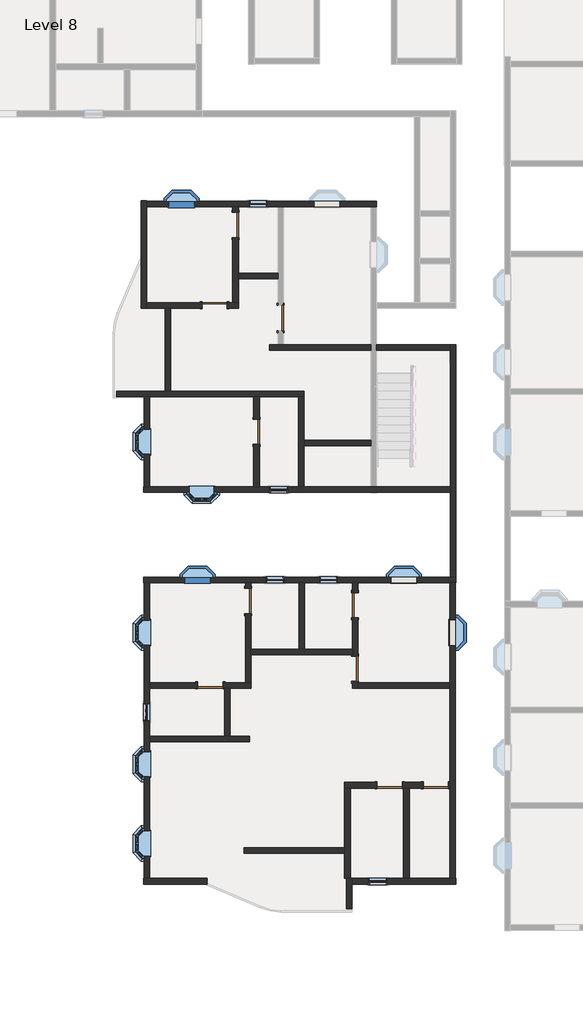
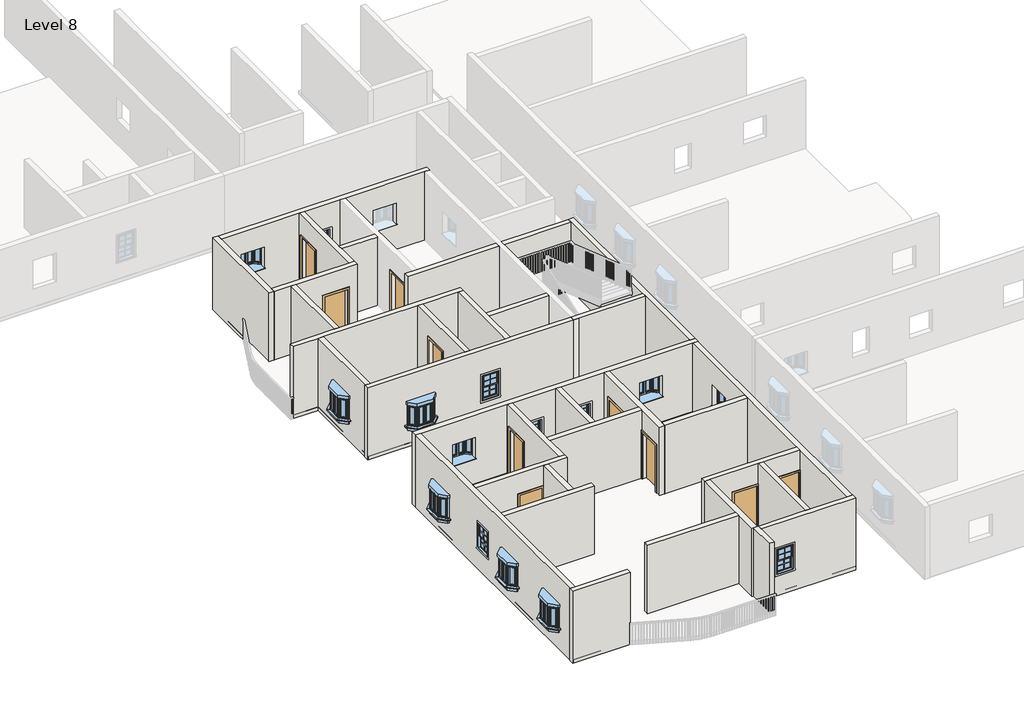
# One storey, part 1 of 14: 33 walls, 15 windows, 10 doors.
"""IFC4 building model written with IfcOpenShell, lengths in millimetres."""

from ifc_helpers import new_model, si_unit, frame, origin, place, context, project, spatial, polyline, outline, extrude, faceted_brep, transform, mapped, element, save
from components import door_54dd4da4, door_719f80de, window_910x910mm_67ef725a, window_8debb0fa

model = new_model("IFC4")

# Units and contexts
model_context = context("Model", 3, world=origin())
ifc_project = project(units=[si_unit("LENGTHUNIT", "METRE", prefix="MILLI")], contexts=[model_context])

# Site, building, storey
site = spatial("IfcSite", under=ifc_project)
building = spatial("IfcBuilding", under=site)
storey = spatial("IfcBuildingStorey", under=building, Name="Level 8", Elevation=21336.0)

# Doors
placement = place(None, origin())
door_shape = door_54dd4da4(model_context)
element("IfcDoor", 1, ObjectType="Single-Flush : 36\" x 84\"", at=placement, inside=storey, context=model_context, shape_type="MappedRepresentation", body=[
    mapped(door_shape, transform((-4626.037215, -17283.4916506, 21336.0), x_axis=(0.0, -1.0, 0.0), y_axis=(1.0, 0.0, 0.0), z_axis=(0.0, 0.0, 1.0))),
])
element("IfcDoor", 2, ObjectType="Single-Flush : 36\" x 84\"", at=placement, inside=storey, context=model_context, shape_type="MappedRepresentation", body=[
    mapped(door_shape, transform((-4626.037215, -14978.4416506, 21336.0), x_axis=(0.0, 1.0, 0.0), y_axis=(-1.0, 0.0, 0.0), z_axis=(0.0, 0.0, 1.0))),
])
element("IfcDoor", 3, ObjectType="Single-Flush : 36\" x 84\"", at=placement, inside=storey, context=model_context, shape_type="MappedRepresentation", body=[
    mapped(door_shape, transform((-9731.437215, -4100.8916506, 21336.0), x_axis=(1.0, 0.0, 0.0), y_axis=(0.0, 1.0, 0.0), z_axis=(0.0, 0.0, 1.0))),
])
element("IfcDoor", 4, ObjectType="Single-Flush : 36\" x 84\"", at=placement, inside=storey, context=model_context, shape_type="MappedRepresentation", body=[
    mapped(door_shape, transform((-7331.137215, -4558.0916506, 21336.0), x_axis=(0.0, -1.0, 0.0), y_axis=(1.0, 0.0, 0.0), z_axis=(0.0, 0.0, 1.0))),
])
door_2_shape = door_719f80de(model_context)
element("IfcDoor", 5, ObjectType="Single-Flush : 36\" x 84\"", at=placement, inside=storey, context=model_context, shape_type="MappedRepresentation", body=[
    mapped(door_2_shape, transform((-9883.837215, -17891.2072331, 21336.0), x_axis=(1.0, 0.0, 0.0), y_axis=(0.0, 1.0, 0.0), z_axis=(0.0, 0.0, 1.0))),
])
element("IfcDoor", 6, ObjectType="Single-Flush : 36\" x 84\"", at=placement, inside=storey, context=model_context, shape_type="MappedRepresentation", body=[
    mapped(door_2_shape, transform((-8512.237215, -14826.0416506, 21336.0), x_axis=(0.0, 1.0, 0.0), y_axis=(-1.0, 0.0, 0.0), z_axis=(0.0, 0.0, 1.0))),
])
element("IfcDoor", 7, ObjectType="Single-Flush : 36\" x 84\"", at=placement, inside=storey, context=model_context, shape_type="MappedRepresentation", body=[
    mapped(door_2_shape, transform((-8207.437215, -8691.9416506, 21336.0), x_axis=(0.0, 1.0, 0.0), y_axis=(-1.0, 0.0, 0.0), z_axis=(0.0, 0.0, 1.0))),
])
element("IfcDoor", 8, ObjectType="Single-Flush : 36\" x 84\"", at=placement, inside=storey, context=model_context, shape_type="MappedRepresentation", body=[
    mapped(door_2_shape, transform((-8969.437215, -1186.2416506, 21336.0), x_axis=(0.0, 1.0, 0.0), y_axis=(-1.0, 0.0, 0.0), z_axis=(0.0, 0.0, 1.0))),
])
element("IfcDoor", 9, ObjectType="Single-Flush : 36\" x 84\"", at=placement, inside=storey, context=model_context, shape_type="MappedRepresentation", body=[
    mapped(door_2_shape, transform((-3374.4891351, -21512.5916506, 21336.0), x_axis=(1.0, 0.0, 0.0), y_axis=(0.0, 1.0, 0.0), z_axis=(0.0, 0.0, 1.0))),
])
element("IfcDoor", 10, ObjectType="Single-Flush : 36\" x 84\"", at=placement, inside=storey, context=model_context, shape_type="MappedRepresentation", body=[
    mapped(door_2_shape, transform((-1698.0891351, -21512.5916506, 21336.0), x_axis=(1.0, 0.0, 0.0), y_axis=(0.0, 1.0, 0.0), z_axis=(0.0, 0.0, 1.0))),
])

# Walls
element("IfcWall", 11, ObjectType="4.5\" p", at=placement, inside=storey, context=model_context, shape_type="Brep", body=[
    faceted_brep([(-9426.637215, -17992.8072331, 23469.6), (-9426.637215, -17992.8072331, 21336.0), (-9375.837215, -17992.8072331, 21336.0), (-9172.637215, -17992.8072331, 21336.0), (-8410.637215, -17992.8072331, 21336.0), (-8410.637215, -17992.8072331, 24384.0), (-9172.637215, -17992.8072331, 24384.0), (-9375.837215, -17992.8072331, 24384.0), (-12087.287215, -17992.8072331, 24384.0), (-12087.287215, -17992.8072331, 21336.0), (-10341.037215, -17992.8072331, 21336.0), (-10341.037215, -17992.8072331, 23469.6), (-8410.637215, -17789.6072331, 21336.0), (-8613.837215, -17789.6072331, 21336.0), (-9426.637215, -17789.6072331, 21336.0), (-9426.637215, -17789.6072331, 23469.6), (-10341.037215, -17789.6072331, 23469.6), (-10341.037215, -17789.6072331, 21336.0), (-12087.287215, -17789.6072331, 21336.0), (-12087.287215, -17789.6072331, 24384.0), (-8613.837215, -17789.6072331, 24384.0), (-8410.637215, -17789.6072331, 24384.0)], [[[0, 1, 2, 3, 4, 5, 6, 7, 8, 9, 10, 11]], [[12, 13, 14, 15, 16, 17, 18, 19, 20, 21]], [[10, 9, 18, 17]], [[4, 3, 2, 1, 14, 13, 12]], [[8, 7, 6, 5, 21, 20, 19]], [[9, 8, 19, 18]], [[5, 4, 12, 21]], [[15, 14, 1, 0]], [[16, 15, 0, 11]], [[17, 16, 11, 10]]]),
])
element("IfcWall", 12, ObjectType="4.5\" p", at=placement, inside=storey, context=model_context, shape_type="Brep", body=[
    faceted_brep([(-8410.637215, -14368.8416506, 23469.6), (-8410.637215, -14368.8416506, 21336.0), (-8410.637215, -14165.6416506, 21336.0), (-8410.637215, -14165.6416506, 24384.0), (-8410.637215, -16572.2916506, 24384.0), (-8410.637215, -16775.4916506, 24384.0), (-8410.637215, -17789.6072331, 24384.0), (-8410.637215, -17789.6072331, 21336.0), (-8410.637215, -16775.4916506, 21336.0), (-8410.637215, -16572.2916506, 21336.0), (-8410.637215, -15283.2416506, 21336.0), (-8410.637215, -15283.2416506, 23469.6), (-8613.837215, -14165.6416506, 21336.0), (-8613.837215, -14368.8416506, 21336.0), (-8613.837215, -14368.8416506, 23469.6), (-8613.837215, -15283.2416506, 23469.6), (-8613.837215, -15283.2416506, 21336.0), (-8613.837215, -17789.6072331, 21336.0), (-8613.837215, -17789.6072331, 24384.0), (-8613.837215, -14165.6416506, 24384.0)], [[[0, 1, 2, 3, 4, 5, 6, 7, 8, 9, 10, 11]], [[12, 13, 14, 15, 16, 17, 18, 19]], [[2, 1, 13, 12]], [[10, 9, 8, 7, 17, 16]], [[6, 5, 4, 3, 19, 18]], [[7, 6, 18, 17]], [[3, 2, 12, 19]], [[14, 13, 1, 0]], [[15, 14, 0, 11]], [[16, 15, 11, 10]]]),
])
element("IfcWall", 13, ObjectType="4.5\" p", at=placement, inside=storey, context=model_context, shape_type="Brep", body=[
    faceted_brep([(-8410.637215, -16775.4916506, 21336.0), (-4727.637215, -16775.4916506, 21336.0), (-4727.637215, -16775.4916506, 24384.0), (-8410.637215, -16775.4916506, 24384.0), (-8410.637215, -16572.2916506, 21336.0), (-8410.637215, -16572.2916506, 24384.0), (-6670.737215, -16572.2916506, 24384.0), (-6467.537215, -16572.2916506, 24384.0), (-4727.637215, -16572.2916506, 24384.0), (-4727.637215, -16572.2916506, 21336.0), (-6467.537215, -16572.2916506, 21336.0), (-6670.737215, -16572.2916506, 21336.0)], [[[0, 1, 2, 3]], [[4, 5, 6, 7, 8, 9, 10, 11]], [[1, 0, 4, 11, 10, 9]], [[3, 2, 8, 7, 6, 5]], [[0, 3, 5, 4]], [[2, 1, 9, 8]]]),
])
element("IfcWall", 14, ObjectType="4.5\" p", at=placement, inside=storey, context=model_context, shape_type="SweptSolid", body=[
    extrude(outline(polyline([(-6670.737215, -16572.2916506), (-6670.737215, -14165.6416506), (-6467.537215, -14165.6416506), (-6467.537215, -16572.2916506), (-6670.737215, -16572.2916506)])), frame((0.0, 0.0, 21336.0), z_axis=(0.0, 0.0, 1.0), x_axis=(1.0, 0.0, 0.0)), (0.0, 0.0, 1.0), 3048.0),
])
element("IfcWall", 15, ObjectType="4.5\" p", at=placement, inside=storey, context=model_context, shape_type="Brep", body=[
    faceted_brep([(-4727.637215, -14165.6416506, 21336.0), (-4727.637215, -14521.2416506, 21336.0), (-4727.637215, -14521.2416506, 23469.6), (-4727.637215, -15435.6416506, 23469.6), (-4727.637215, -15435.6416506, 21336.0), (-4727.637215, -16572.2916506, 21336.0), (-4727.637215, -16775.4916506, 21336.0), (-4727.637215, -16826.2916506, 21336.0), (-4727.637215, -16826.2916506, 23469.6), (-4727.637215, -17740.6916506, 23469.6), (-4727.637215, -17740.6916506, 21336.0), (-4727.637215, -17994.6916506, 21336.0), (-4727.637215, -17994.6916506, 24384.0), (-4727.637215, -16775.4916506, 24384.0), (-4727.637215, -16572.2916506, 24384.0), (-4727.637215, -14165.6416506, 24384.0), (-4524.437215, -14521.2416506, 23469.6), (-4524.437215, -14521.2416506, 21336.0), (-4524.437215, -14165.6416506, 21336.0), (-4524.437215, -14165.6416506, 24384.0), (-4524.437215, -17791.4916506, 24384.0), (-4524.437215, -17994.6916506, 24384.0), (-4524.437215, -17994.6916506, 21336.0), (-4524.437215, -17791.4916506, 21336.0), (-4524.437215, -17740.6916506, 21336.0), (-4524.437215, -17740.6916506, 23469.6), (-4524.437215, -16826.2916506, 23469.6), (-4524.437215, -16826.2916506, 21336.0), (-4524.437215, -15435.6416506, 21336.0), (-4524.437215, -15435.6416506, 23469.6)], [[[0, 1, 2, 3, 4, 5, 6, 7, 8, 9, 10, 11, 12, 13, 14, 15]], [[16, 17, 18, 19, 20, 21, 22, 23, 24, 25, 26, 27, 28, 29]], [[11, 10, 24, 23, 22]], [[28, 27, 7, 6, 5, 4]], [[18, 17, 1, 0]], [[15, 14, 13, 12, 21, 20, 19]], [[0, 15, 19, 18]], [[12, 11, 22, 21]], [[25, 24, 10, 9]], [[26, 25, 9, 8]], [[27, 26, 8, 7]], [[2, 1, 17, 16]], [[3, 2, 16, 29]], [[4, 3, 29, 28]]]),
])
element("IfcWall", 16, ObjectType="4.5\" p", at=placement, inside=storey, context=model_context, shape_type="SweptSolid", body=[
    extrude(outline(polyline([(-4524.437215, -17791.4916506), (-1190.0891351, -17791.4916506), (-1190.0891351, -17994.6916506), (-4524.437215, -17994.6916506), (-4524.437215, -17791.4916506)])), frame((0.0, 0.0, 21336.0), z_axis=(0.0, 0.0, 1.0), x_axis=(1.0, 0.0, 0.0)), (0.0, 0.0, 1.0), 3048.0),
])
element("IfcWall", 17, ObjectType="4.5\" p", at=placement, inside=storey, context=model_context, shape_type="SweptSolid", body=[
    extrude(outline(polyline([(-9375.837215, -19734.5916506), (-9375.837215, -17992.8072331), (-9172.637215, -17992.8072331), (-9172.637215, -19734.5916506), (-9375.837215, -19734.5916506)])), frame((0.0, 0.0, 21336.0), z_axis=(0.0, 0.0, 1.0), x_axis=(1.0, 0.0, 0.0)), (0.0, 0.0, 1.0), 3048.0),
])
element("IfcWall", 18, ObjectType="4.5\" p", at=placement, inside=storey, context=model_context, shape_type="Brep", body=[
    faceted_brep([(-12087.287215, -19937.7916506, 21336.0), (-8455.087215, -19937.7916506, 21336.0), (-8455.087215, -19937.7916506, 24384.0), (-12087.287215, -19937.7916506, 24384.0), (-12087.287215, -19734.5916506, 21336.0), (-12087.287215, -19734.5916506, 24384.0), (-9375.837215, -19734.5916506, 24384.0), (-9172.637215, -19734.5916506, 24384.0), (-8455.087215, -19734.5916506, 24384.0), (-8455.087215, -19734.5916506, 21336.0), (-9172.637215, -19734.5916506, 21336.0), (-9375.837215, -19734.5916506, 21336.0)], [[[0, 1, 2, 3]], [[4, 5, 6, 7, 8, 9, 10, 11]], [[1, 0, 4, 11, 10, 9]], [[2, 1, 9, 8]], [[3, 2, 8, 7, 6, 5]], [[0, 3, 5, 4]]]),
])
element("IfcWall", 19, ObjectType="4.5\" p", at=placement, inside=storey, context=model_context, shape_type="Brep", body=[
    faceted_brep([(-13293.787215, -7421.9416506, 21336.0), (-12290.487215, -7421.9416506, 21336.0), (-12087.287215, -7421.9416506, 21336.0), (-8309.037215, -7421.9416506, 21336.0), (-8105.837215, -7421.9416506, 21336.0), (-6689.787215, -7421.9416506, 21336.0), (-6486.587215, -7421.9416506, 21336.0), (-6486.587215, -7421.9416506, 24384.0), (-6689.787215, -7421.9416506, 24384.0), (-8105.837215, -7421.9416506, 24384.0), (-8309.037215, -7421.9416506, 24384.0), (-12087.287215, -7421.9416506, 24384.0), (-12290.487215, -7421.9416506, 24384.0), (-13293.787215, -7421.9416506, 24384.0), (-13293.787215, -7218.7416506, 21336.0), (-13293.787215, -7218.7416506, 24384.0), (-11528.487215, -7218.7416506, 24384.0), (-11325.287215, -7218.7416506, 24384.0), (-6486.587215, -7218.7416506, 24384.0), (-6486.587215, -7218.7416506, 21336.0), (-11325.287215, -7218.7416506, 21336.0), (-11528.487215, -7218.7416506, 21336.0)], [[[0, 1, 2, 3, 4, 5, 6, 7, 8, 9, 10, 11, 12, 13]], [[14, 15, 16, 17, 18, 19, 20, 21]], [[6, 5, 4, 3, 2, 1, 0, 14, 21, 20, 19]], [[13, 12, 11, 10, 9, 8, 7, 18, 17, 16, 15]], [[0, 13, 15, 14]], [[7, 6, 19, 18]]]),
])
element("IfcWall", 20, ObjectType="4.5\" p", at=placement, inside=storey, context=model_context, shape_type="Brep", body=[
    faceted_brep([(-12201.587215, -4202.4916506, 21336.0), (-12201.587215, -3999.2916506, 21336.0), (-12201.587215, -525.8416506, 21336.0), (-12201.587215, -322.6416506, 21336.0), (-12201.587215, -309.9416506, 21336.0), (-12201.587215, -309.9416506, 24384.0), (-12201.587215, -322.6416506, 24384.0), (-12201.587215, -525.8416506, 24384.0), (-12201.587215, -3999.2916506, 24384.0), (-12201.587215, -4202.4916506, 24384.0), (-12404.787215, -4202.4916506, 21336.0), (-12404.787215, -4202.4916506, 24384.0), (-12404.787215, -309.9416506, 24384.0), (-12404.787215, -309.9416506, 21336.0)], [[[0, 1, 2, 3, 4, 5, 6, 7, 8, 9]], [[10, 11, 12, 13]], [[4, 3, 2, 1, 0, 10, 13]], [[5, 4, 13, 12]], [[9, 8, 7, 6, 5, 12, 11]], [[0, 9, 11, 10]]]),
])
element("IfcWall", 21, ObjectType="4.5\" p", at=placement, inside=storey, context=model_context, shape_type="Brep", body=[
    faceted_brep([(-9274.237215, -4202.4916506, 23469.6), (-9274.237215, -4202.4916506, 21336.0), (-8867.837215, -4202.4916506, 21336.0), (-8867.837215, -4202.4916506, 24384.0), (-11325.287215, -4202.4916506, 24384.0), (-11528.487215, -4202.4916506, 24384.0), (-12201.587215, -4202.4916506, 24384.0), (-12201.587215, -4202.4916506, 21336.0), (-11528.487215, -4202.4916506, 21336.0), (-11325.287215, -4202.4916506, 21336.0), (-10188.637215, -4202.4916506, 21336.0), (-10188.637215, -4202.4916506, 23469.6), (-8867.837215, -3999.2916506, 21336.0), (-9071.037215, -3999.2916506, 21336.0), (-9274.237215, -3999.2916506, 21336.0), (-9274.237215, -3999.2916506, 23469.6), (-10188.637215, -3999.2916506, 23469.6), (-10188.637215, -3999.2916506, 21336.0), (-12201.587215, -3999.2916506, 21336.0), (-12201.587215, -3999.2916506, 24384.0), (-9071.037215, -3999.2916506, 24384.0), (-8867.837215, -3999.2916506, 24384.0)], [[[0, 1, 2, 3, 4, 5, 6, 7, 8, 9, 10, 11]], [[12, 13, 14, 15, 16, 17, 18, 19, 20, 21]], [[2, 1, 14, 13, 12]], [[10, 9, 8, 7, 18, 17]], [[6, 5, 4, 3, 21, 20, 19]], [[7, 6, 19, 18]], [[3, 2, 12, 21]], [[15, 14, 1, 0]], [[16, 15, 0, 11]], [[17, 16, 11, 10]]]),
])
element("IfcWall", 22, ObjectType="4.5\" p", at=placement, inside=storey, context=model_context, shape_type="Brep", body=[
    faceted_brep([(-8867.837215, -729.0416506, 23469.6), (-8867.837215, -729.0416506, 21336.0), (-8867.837215, -525.8416506, 21336.0), (-8867.837215, -525.8416506, 24384.0), (-8867.837215, -2932.4916506, 24384.0), (-8867.837215, -3135.6916506, 24384.0), (-8867.837215, -3999.2916506, 24384.0), (-8867.837215, -3999.2916506, 21336.0), (-8867.837215, -3135.6916506, 21336.0), (-8867.837215, -2932.4916506, 21336.0), (-8867.837215, -1643.4416506, 21336.0), (-8867.837215, -1643.4416506, 23469.6), (-9071.037215, -525.8416506, 21336.0), (-9071.037215, -729.0416506, 21336.0), (-9071.037215, -729.0416506, 23469.6), (-9071.037215, -1643.4416506, 23469.6), (-9071.037215, -1643.4416506, 21336.0), (-9071.037215, -3999.2916506, 21336.0), (-9071.037215, -3999.2916506, 24384.0), (-9071.037215, -525.8416506, 24384.0)], [[[0, 1, 2, 3, 4, 5, 6, 7, 8, 9, 10, 11]], [[12, 13, 14, 15, 16, 17, 18, 19]], [[2, 1, 13, 12]], [[10, 9, 8, 7, 17, 16]], [[6, 5, 4, 3, 19, 18]], [[7, 6, 18, 17]], [[3, 2, 12, 19]], [[14, 13, 1, 0]], [[15, 14, 0, 11]], [[16, 15, 11, 10]]]),
])
element("IfcWall", 23, ObjectType="4.5\" p", at=placement, inside=storey, context=model_context, shape_type="SweptSolid", body=[
    extrude(outline(polyline([(-7432.737215, -3135.6916506), (-8867.837215, -3135.6916506), (-8867.837215, -2932.4916506), (-7432.737215, -2932.4916506), (-7432.737215, -3135.6916506)])), frame((0.0, 0.0, 21336.0), z_axis=(0.0, 0.0, 1.0), x_axis=(1.0, 0.0, 0.0)), (0.0, 0.0, 1.0), 3048.0),
])
element("IfcWall", 24, ObjectType="4.5\" p", at=placement, inside=storey, context=model_context, shape_type="Brep", body=[
    faceted_brep([(-7731.187215, -5726.4916506, 24384.0), (-7731.187215, -5726.4916506, 21336.0), (-4060.887215, -5726.4916506, 21336.0), (-4060.887215, -5726.4916506, 24384.0), (-7731.187215, -5523.2916506, 21336.0), (-7731.187215, -5523.2916506, 24384.0), (-7432.737215, -5523.2916506, 24384.0), (-7229.537215, -5523.2916506, 24384.0), (-4060.887215, -5523.2916506, 24384.0), (-4060.887215, -5523.2916506, 21336.0), (-7229.537215, -5523.2916506, 21336.0), (-7432.737215, -5523.2916506, 21336.0)], [[[0, 1, 2, 3]], [[4, 5, 6, 7, 8, 9, 10, 11]], [[1, 4, 11, 10, 9, 2]], [[5, 0, 3, 8, 7, 6]], [[1, 0, 5, 4]], [[3, 2, 9, 8]]]),
    faceted_brep([(-1177.3891351, -5726.4916506, 21336.0), (-1177.3891351, -5726.4916506, 24384.0), (-3857.687215, -5726.4916506, 24384.0), (-3857.687215, -5726.4916506, 21336.0), (-1177.3891351, -5523.2916506, 24384.0), (-1177.3891351, -5523.2916506, 21336.0), (-3857.687215, -5523.2916506, 21336.0), (-3857.687215, -5523.2916506, 24384.0)], [[[0, 1, 2, 3]], [[4, 5, 6, 7]], [[5, 0, 3, 6]], [[1, 4, 7, 2]], [[1, 0, 5, 4]], [[3, 2, 7, 6]]]),
])
element("IfcWall", 25, ObjectType="4.5\" p", at=placement, inside=storey, context=model_context, shape_type="SweptSolid", body=[
    extrude(outline(polyline([(-11528.487215, -7218.7416506), (-11528.487215, -4202.4916506), (-11325.287215, -4202.4916506), (-11325.287215, -7218.7416506), (-11528.487215, -7218.7416506)])), frame((0.0, 0.0, 21336.0), z_axis=(0.0, 0.0, 1.0), x_axis=(1.0, 0.0, 0.0)), (0.0, 0.0, 1.0), 3048.0),
])
element("IfcWall", 26, ObjectType="4.5\" p", at=placement, inside=storey, context=model_context, shape_type="SweptSolid", body=[
    extrude(outline(polyline([(-7421.9416506, 21336.0), (-8234.7416506, 21336.0), (-8234.7416506, 23469.6), (-9149.1416506, 23469.6), (-9149.1416506, 21336.0), (-10685.8416506, 21336.0), (-10685.8416506, 24384.0), (-7421.9416506, 24384.0), (-7421.9416506, 21336.0)])), frame((-8309.037215, 0.0, 0.0), z_axis=(1.0, 0.0, 0.0), x_axis=(0.0, 1.0, 0.0)), (0.0, 0.0, 1.0), 203.2),
])
element("IfcWall", 27, ObjectType="4.5\" p", at=placement, inside=storey, context=model_context, shape_type="Brep", body=[
    faceted_brep([(-6689.787215, -7421.9416506, 21336.0), (-6689.787215, -10685.8416506, 21336.0), (-6689.787215, -10685.8416506, 24384.0), (-6689.787215, -7421.9416506, 24384.0), (-6486.587215, -7421.9416506, 21336.0), (-6486.587215, -7421.9416506, 24384.0), (-6486.587215, -8990.3916506, 24384.0), (-6486.587215, -9193.5916506, 24384.0), (-6486.587215, -10685.8416506, 24384.0), (-6486.587215, -10685.8416506, 21336.0), (-6486.587215, -9193.5916506, 21336.0), (-6486.587215, -8990.3916506, 21336.0)], [[[0, 1, 2, 3]], [[4, 5, 6, 7, 8, 9, 10, 11]], [[1, 0, 4, 11, 10, 9]], [[3, 2, 8, 7, 6, 5]], [[0, 3, 5, 4]], [[2, 1, 9, 8]]]),
])
element("IfcWall", 28, ObjectType="4.5\" p", at=placement, inside=storey, context=model_context, shape_type="SweptSolid", body=[
    extrude(outline(polyline([(-4060.887215, -9193.5916506), (-6486.587215, -9193.5916506), (-6486.587215, -8990.3916506), (-4060.887215, -8990.3916506), (-4060.887215, -9193.5916506)])), frame((0.0, 0.0, 21336.0), z_axis=(0.0, 0.0, 1.0), x_axis=(1.0, 0.0, 0.0)), (0.0, 0.0, 1.0), 3048.0),
])
element("IfcWall", 29, ObjectType="9\"", at=placement, inside=storey, context=model_context, shape_type="SweptSolid", body=[
    extrude(outline(polyline([(-5006.4391351, -23982.7416506), (-8664.637215, -23982.7416506), (-8664.637215, -23779.5416506), (-5006.4391351, -23779.5416506), (-5006.4391351, -23982.7416506)])), frame((0.0, 0.0, 21336.0), z_axis=(0.0, 0.0, 1.0), x_axis=(1.0, 0.0, 0.0)), (0.0, 0.0, 1.0), 3048.0),
])
element("IfcWall", 30, ObjectType="9\"", at=placement, inside=storey, context=model_context, shape_type="Brep", body=[
    faceted_brep([(-1190.0891351, -21410.9916506, 21336.0), (-1240.8891351, -21410.9916506, 21336.0), (-1240.8891351, -21410.9916506, 23469.6), (-2155.2891351, -21410.9916506, 23469.6), (-2155.2891351, -21410.9916506, 21336.0), (-2917.2891351, -21410.9916506, 21336.0), (-2917.2891351, -21410.9916506, 23469.6), (-3831.6891351, -21410.9916506, 23469.6), (-3831.6891351, -21410.9916506, 21336.0), (-5006.4391351, -21410.9916506, 21336.0), (-5006.4391351, -21410.9916506, 24384.0), (-1190.0891351, -21410.9916506, 24384.0), (-1240.8891351, -21614.1916506, 23469.6), (-1240.8891351, -21614.1916506, 21336.0), (-1190.0891351, -21614.1916506, 21336.0), (-1190.0891351, -21614.1916506, 24384.0), (-2663.2891351, -21614.1916506, 24384.0), (-2866.4891351, -21614.1916506, 24384.0), (-4803.2391351, -21614.1916506, 24384.0), (-5006.4391351, -21614.1916506, 24384.0), (-5006.4391351, -21614.1916506, 21336.0), (-4803.2391351, -21614.1916506, 21336.0), (-3831.6891351, -21614.1916506, 21336.0), (-3831.6891351, -21614.1916506, 23469.6), (-2917.2891351, -21614.1916506, 23469.6), (-2917.2891351, -21614.1916506, 21336.0), (-2866.4891351, -21614.1916506, 21336.0), (-2663.2891351, -21614.1916506, 21336.0), (-2155.2891351, -21614.1916506, 21336.0), (-2155.2891351, -21614.1916506, 23469.6)], [[[0, 1, 2, 3, 4, 5, 6, 7, 8, 9, 10, 11]], [[12, 13, 14, 15, 16, 17, 18, 19, 20, 21, 22, 23, 24, 25, 26, 27, 28, 29]], [[22, 21, 20, 9, 8]], [[14, 13, 1, 0]], [[28, 27, 26, 25, 5, 4]], [[11, 10, 19, 18, 17, 16, 15]], [[0, 11, 15, 14]], [[10, 9, 20, 19]], [[6, 5, 25, 24]], [[7, 6, 24, 23]], [[8, 7, 23, 22]], [[2, 1, 13, 12]], [[3, 2, 12, 29]], [[4, 3, 29, 28]]]),
])
element("IfcWall", 31, ObjectType="9\"", at=placement, inside=storey, context=model_context, shape_type="Brep", body=[
    faceted_brep([(-5006.4391351, -21614.1916506, 21336.0), (-5006.4391351, -23779.5416506, 21336.0), (-5006.4391351, -23982.7416506, 21336.0), (-5006.4391351, -24897.1416506, 21336.0), (-5006.4391351, -24897.1416506, 24384.0), (-5006.4391351, -23982.7416506, 24384.0), (-5006.4391351, -23779.5416506, 24384.0), (-5006.4391351, -21614.1916506, 24384.0), (-4803.2391351, -21614.1916506, 21336.0), (-4803.2391351, -21614.1916506, 24384.0), (-4803.2391351, -24897.1416506, 24384.0), (-4803.2391351, -24897.1416506, 21336.0), (-4949.2891351, -24897.1416506, 21336.0), (-4949.2891351, -24897.1416506, 24384.0)], [[[0, 1, 2, 3, 4, 5, 6, 7]], [[8, 9, 10, 11]], [[3, 2, 1, 0, 8, 11, 12]], [[7, 6, 5, 4, 13, 10, 9]], [[0, 7, 9, 8]], [[4, 3, 12, 11, 10, 13]]]),
])
element("IfcWall", 32, ObjectType="9\"", at=placement, inside=storey, context=model_context, shape_type="SweptSolid", body=[
    extrude(outline(polyline([(-2866.4891351, -24897.1416506), (-2866.4891351, -21614.1916506), (-2663.2891351, -21614.1916506), (-2663.2891351, -24897.1416506), (-2866.4891351, -24897.1416506)])), frame((0.0, 0.0, 21336.0), z_axis=(0.0, 0.0, 1.0), x_axis=(1.0, 0.0, 0.0)), (0.0, 0.0, 1.0), 3048.0),
])
element("IfcWall", 33, ObjectType="9\"", at=placement, inside=storey, context=model_context, shape_type="SweptSolid", body=[
    extrude(outline(polyline([(-5006.4391351, -23982.7416506), (-8664.637215, -23982.7416506), (-8664.637215, -23779.5416506), (-5006.4391351, -23779.5416506), (-5006.4391351, -23982.7416506)])), frame((0.0, 0.0, 21336.0), z_axis=(0.0, 0.0, 1.0), x_axis=(1.0, 0.0, 0.0)), (0.0, 0.0, 1.0), 3048.0),
])
element("IfcWall", 34, ObjectType="9\" w", at=placement, inside=storey, context=model_context, shape_type="Brep", body=[
    faceted_brep([(-12303.187215, -14165.6416506, 21336.0), (-12290.487215, -14165.6416506, 21336.0), (-12087.287215, -14165.6416506, 21336.0), (-8613.837215, -14165.6416506, 21336.0), (-8410.637215, -14165.6416506, 21336.0), (-6670.737215, -14165.6416506, 21336.0), (-6467.537215, -14165.6416506, 21336.0), (-4727.637215, -14165.6416506, 21336.0), (-4524.437215, -14165.6416506, 21336.0), (-1190.0891351, -14165.6416506, 21336.0), (-986.8891351, -14165.6416506, 21336.0), (-961.4891351, -14165.6416506, 21336.0), (-961.4891351, -14165.6416506, 24384.0), (-986.8891351, -14165.6416506, 24384.0), (-1190.0891351, -14165.6416506, 24384.0), (-4524.437215, -14165.6416506, 24384.0), (-4727.637215, -14165.6416506, 24384.0), (-6467.537215, -14165.6416506, 24384.0), (-6670.737215, -14165.6416506, 24384.0), (-8410.637215, -14165.6416506, 24384.0), (-8613.837215, -14165.6416506, 24384.0), (-12087.287215, -14165.6416506, 24384.0), (-12290.487215, -14165.6416506, 24384.0), (-12303.187215, -14165.6416506, 24384.0), (-10805.562215, -14165.6416506, 23446.0), (-9895.562215, -14165.6416506, 23446.0), (-9895.562215, -14165.6416506, 22536.0), (-10805.562215, -14165.6416506, 22536.0), (-3312.2631751, -14165.6416506, 23446.0), (-2402.2631751, -14165.6416506, 23446.0), (-2402.2631751, -14165.6416506, 22536.0), (-3312.2631751, -14165.6416506, 22536.0), (-7870.887215, -14165.6416506, 23317.2), (-7210.487215, -14165.6416506, 23317.2), (-7210.487215, -14165.6416506, 22250.4), (-7870.887215, -14165.6416506, 22250.4), (-5927.787215, -14165.6416506, 23317.2), (-5267.387215, -14165.6416506, 23317.2), (-5267.387215, -14165.6416506, 22250.4), (-5927.787215, -14165.6416506, 22250.4), (-12303.187215, -13962.4416506, 21336.0), (-12303.187215, -13962.4416506, 24384.0), (-1177.3891351, -13962.4416506, 24384.0), (-974.1891351, -13962.4416506, 24384.0), (-961.4891351, -13962.4416506, 24384.0), (-961.4891351, -13962.4416506, 21336.0), (-974.1891351, -13962.4416506, 21336.0), (-1177.3891351, -13962.4416506, 21336.0), (-10805.562215, -13962.4416506, 23446.0), (-10805.562215, -13962.4416506, 22536.0), (-9895.562215, -13962.4416506, 22536.0), (-9895.562215, -13962.4416506, 23446.0), (-3312.2631751, -13962.4416506, 23446.0), (-3312.2631751, -13962.4416506, 22536.0), (-2402.2631751, -13962.4416506, 22536.0), (-2402.2631751, -13962.4416506, 23446.0), (-7870.887215, -13962.4416506, 23317.2), (-7870.887215, -13962.4416506, 22250.4), (-7210.487215, -13962.4416506, 22250.4), (-7210.487215, -13962.4416506, 23317.2), (-5927.787215, -13962.4416506, 23317.2), (-5927.787215, -13962.4416506, 22250.4), (-5267.387215, -13962.4416506, 22250.4), (-5267.387215, -13962.4416506, 23317.2)], [[[0, 1, 2, 3, 4, 5, 6, 7, 8, 9, 10, 11, 12, 13, 14, 15, 16, 17, 18, 19, 20, 21, 22, 23], [24, 25, 26, 27], [28, 29, 30, 31], [32, 33, 34, 35], [36, 37, 38, 39]], [[40, 41, 42, 43, 44, 45, 46, 47], [48, 49, 50, 51], [52, 53, 54, 55], [56, 57, 58, 59], [60, 61, 62, 63]], [[11, 10, 9, 8, 7, 6, 5, 4, 3, 2, 1, 0, 40, 47, 46, 45]], [[12, 11, 45, 44]], [[23, 22, 21, 20, 19, 18, 17, 16, 15, 14, 13, 12, 44, 43, 42, 41]], [[0, 23, 41, 40]], [[49, 48, 24, 27]], [[50, 49, 27, 26]], [[51, 50, 26, 25]], [[48, 51, 25, 24]], [[53, 52, 28, 31]], [[54, 53, 31, 30]], [[55, 54, 30, 29]], [[52, 55, 29, 28]], [[57, 56, 32, 35]], [[58, 57, 35, 34]], [[59, 58, 34, 33]], [[56, 59, 33, 32]], [[61, 60, 36, 39]], [[62, 61, 39, 38]], [[63, 62, 38, 37]], [[60, 63, 37, 36]]]),
])
element("IfcWall", 35, ObjectType="9\" w", at=placement, inside=storey, context=model_context, shape_type="Brep", body=[
    faceted_brep([(-10004.0323936, -24897.1416506, 21336.0), (-12087.287215, -24897.1416506, 21336.0), (-12290.487215, -24897.1416506, 21336.0), (-12303.187215, -24897.1416506, 21336.0), (-12303.187215, -24897.1416506, 24384.0), (-12290.487215, -24897.1416506, 24384.0), (-12087.287215, -24897.1416506, 24384.0), (-10004.0323936, -24897.1416506, 24384.0), (-10004.0323936, -25100.3416506, 21336.0), (-10004.0323936, -25100.3416506, 24384.0), (-12303.187215, -25100.3416506, 24384.0), (-12303.187215, -25100.3416506, 21336.0)], [[[0, 1, 2, 3, 4, 5, 6, 7]], [[8, 9, 10, 11]], [[3, 2, 1, 0, 8, 11]], [[4, 3, 11, 10]], [[7, 6, 5, 4, 10, 9]], [[0, 7, 9, 8]]]),
])
element("IfcWall", 36, ObjectType="9\" w", at=placement, inside=storey, context=model_context, shape_type="Brep", body=[
    faceted_brep([(-4746.0891351, -25989.3416506, 21336.0), (-4746.0891351, -25100.3416506, 21336.0), (-4746.0891351, -24897.1416506, 21336.0), (-4746.0891351, -24897.1416506, 24384.0), (-4746.0891351, -25100.3416506, 24384.0), (-4746.0891351, -25989.3416506, 24384.0), (-4949.2891351, -25989.3416506, 21336.0), (-4949.2891351, -25989.3416506, 24384.0), (-4949.2891351, -24897.1416506, 24384.0), (-4949.2891351, -24897.1416506, 21336.0), (-4803.2391351, -24897.1416506, 21336.0), (-4803.2391351, -24897.1416506, 24384.0)], [[[0, 1, 2, 3, 4, 5]], [[6, 7, 8, 9]], [[2, 1, 0, 6, 9, 10]], [[5, 4, 3, 11, 8, 7]], [[0, 5, 7, 6]], [[3, 2, 10, 9, 8, 11]]]),
])
element("IfcWall", 37, ObjectType="9\" w", at=placement, inside=storey, context=model_context, shape_type="Brep", body=[
    faceted_brep([(-4746.0891351, -25100.3416506, 21336.0), (-961.4891351, -25100.3416506, 21336.0), (-961.4891351, -25100.3416506, 24384.0), (-4746.0891351, -25100.3416506, 24384.0), (-3476.0891351, -25100.3416506, 23317.2), (-3476.0891351, -25100.3416506, 22250.4), (-4136.4891351, -25100.3416506, 22250.4), (-4136.4891351, -25100.3416506, 23317.2), (-4746.0891351, -24897.1416506, 21336.0), (-4746.0891351, -24897.1416506, 24384.0), (-2866.4891351, -24897.1416506, 24384.0), (-2663.2891351, -24897.1416506, 24384.0), (-1190.0891351, -24897.1416506, 24384.0), (-986.8891351, -24897.1416506, 24384.0), (-961.4891351, -24897.1416506, 24384.0), (-961.4891351, -24897.1416506, 21336.0), (-986.8891351, -24897.1416506, 21336.0), (-1190.0891351, -24897.1416506, 21336.0), (-2663.2891351, -24897.1416506, 21336.0), (-2866.4891351, -24897.1416506, 21336.0), (-3476.0891351, -24897.1416506, 23317.2), (-4136.4891351, -24897.1416506, 23317.2), (-4136.4891351, -24897.1416506, 22250.4), (-3476.0891351, -24897.1416506, 22250.4)], [[[0, 1, 2, 3], [4, 5, 6, 7]], [[8, 9, 10, 11, 12, 13, 14, 15, 16, 17, 18, 19], [20, 21, 22, 23]], [[1, 0, 8, 19, 18, 17, 16, 15]], [[2, 1, 15, 14]], [[3, 2, 14, 13, 12, 11, 10, 9]], [[0, 3, 9, 8]], [[5, 4, 20, 23]], [[6, 5, 23, 22]], [[7, 6, 22, 21]], [[4, 7, 21, 20]]]),
])
element("IfcWall", 38, ObjectType="9\" w", at=placement, inside=storey, context=model_context, shape_type="Brep", body=[
    faceted_brep([(-12290.487215, -14165.6416506, 21336.0), (-12290.487215, -24897.1416506, 21336.0), (-12290.487215, -24897.1416506, 24384.0), (-12290.487215, -14165.6416506, 24384.0), (-12290.487215, -16432.6244419, 23160.4), (-12290.487215, -16432.6244419, 22250.4), (-12290.487215, -15522.6244419, 22250.4), (-12290.487215, -15522.6244419, 23160.4), (-12290.487215, -21205.5916506, 23160.4), (-12290.487215, -21205.5916506, 22250.4), (-12290.487215, -20295.5916506, 22250.4), (-12290.487215, -20295.5916506, 23160.4), (-12290.487215, -24082.1416506, 23160.4), (-12290.487215, -24082.1416506, 22250.4), (-12290.487215, -23172.1416506, 22250.4), (-12290.487215, -23172.1416506, 23160.4), (-12290.487215, -19193.8994419, 23317.2), (-12290.487215, -19193.8994419, 22250.4), (-12290.487215, -18533.4994419, 22250.4), (-12290.487215, -18533.4994419, 23317.2), (-12087.287215, -14165.6416506, 21336.0), (-12087.287215, -14165.6416506, 24384.0), (-12087.287215, -17789.6072331, 24384.0), (-12087.287215, -17992.8072331, 24384.0), (-12087.287215, -19734.5916506, 24384.0), (-12087.287215, -19937.7916506, 24384.0), (-12087.287215, -24897.1416506, 24384.0), (-12087.287215, -24897.1416506, 21336.0), (-12087.287215, -19937.7916506, 21336.0), (-12087.287215, -19734.5916506, 21336.0), (-12087.287215, -17992.8072331, 21336.0), (-12087.287215, -17789.6072331, 21336.0), (-12087.287215, -16432.6244419, 23160.4), (-12087.287215, -15522.6244419, 23160.4), (-12087.287215, -15522.6244419, 22250.4), (-12087.287215, -16432.6244419, 22250.4), (-12087.287215, -21205.5916506, 23160.4), (-12087.287215, -20295.5916506, 23160.4), (-12087.287215, -20295.5916506, 22250.4), (-12087.287215, -21205.5916506, 22250.4), (-12087.287215, -24082.1416506, 23160.4), (-12087.287215, -23172.1416506, 23160.4), (-12087.287215, -23172.1416506, 22250.4), (-12087.287215, -24082.1416506, 22250.4), (-12087.287215, -19193.8994419, 23317.2), (-12087.287215, -18533.4994419, 23317.2), (-12087.287215, -18533.4994419, 22250.4), (-12087.287215, -19193.8994419, 22250.4)], [[[0, 1, 2, 3], [4, 5, 6, 7], [8, 9, 10, 11], [12, 13, 14, 15], [16, 17, 18, 19]], [[20, 21, 22, 23, 24, 25, 26, 27, 28, 29, 30, 31], [32, 33, 34, 35], [36, 37, 38, 39], [40, 41, 42, 43], [44, 45, 46, 47]], [[1, 0, 20, 31, 30, 29, 28, 27]], [[3, 2, 26, 25, 24, 23, 22, 21]], [[0, 3, 21, 20]], [[2, 1, 27, 26]], [[5, 4, 32, 35]], [[6, 5, 35, 34]], [[7, 6, 34, 33]], [[4, 7, 33, 32]], [[9, 8, 36, 39]], [[10, 9, 39, 38]], [[11, 10, 38, 37]], [[8, 11, 37, 36]], [[13, 12, 40, 43]], [[14, 13, 43, 42]], [[15, 14, 42, 41]], [[12, 15, 41, 40]], [[17, 16, 44, 47]], [[18, 17, 47, 46]], [[19, 18, 46, 45]], [[16, 19, 45, 44]]]),
])
element("IfcWall", 39, ObjectType="9\" w", at=placement, inside=storey, context=model_context, shape_type="Brep", body=[
    faceted_brep([(-1190.0891351, -14165.6416506, 21336.0), (-1190.0891351, -17791.4916506, 21336.0), (-1190.0891351, -17994.6916506, 21336.0), (-1190.0891351, -21410.9916506, 21336.0), (-1190.0891351, -21614.1916506, 21336.0), (-1190.0891351, -24897.1416506, 21336.0), (-1190.0891351, -24897.1416506, 24384.0), (-1190.0891351, -21614.1916506, 24384.0), (-1190.0891351, -21410.9916506, 24384.0), (-1190.0891351, -17994.6916506, 24384.0), (-1190.0891351, -17791.4916506, 24384.0), (-1190.0891351, -14165.6416506, 24384.0), (-1190.0891351, -15523.5666506, 23446.0), (-1190.0891351, -16433.5666506, 23446.0), (-1190.0891351, -16433.5666506, 22536.0), (-1190.0891351, -15523.5666506, 22536.0), (-986.8891351, -14165.6416506, 21336.0), (-986.8891351, -14165.6416506, 24384.0), (-986.8891351, -24897.1416506, 24384.0), (-986.8891351, -24897.1416506, 21336.0), (-986.8891351, -15523.5666506, 23446.0), (-986.8891351, -15523.5666506, 22536.0), (-986.8891351, -16433.5666506, 22536.0), (-986.8891351, -16433.5666506, 23446.0)], [[[0, 1, 2, 3, 4, 5, 6, 7, 8, 9, 10, 11], [12, 13, 14, 15]], [[16, 17, 18, 19], [20, 21, 22, 23]], [[5, 4, 3, 2, 1, 0, 16, 19]], [[11, 10, 9, 8, 7, 6, 18, 17]], [[0, 11, 17, 16]], [[6, 5, 19, 18]], [[21, 20, 12, 15]], [[22, 21, 15, 14]], [[23, 22, 14, 13]], [[20, 23, 13, 12]]]),
])
element("IfcWall", 40, ObjectType="9\" w", at=placement, inside=storey, context=model_context, shape_type="Brep", body=[
    faceted_brep([(-1177.3891351, -5523.2916506, 21336.0), (-1177.3891351, -5726.4916506, 21336.0), (-1177.3891351, -10685.8416506, 21336.0), (-1177.3891351, -10889.0416506, 21336.0), (-1177.3891351, -13962.4416506, 21336.0), (-1177.3891351, -13962.4416506, 24384.0), (-1177.3891351, -10889.0416506, 24384.0), (-1177.3891351, -10685.8416506, 24384.0), (-1177.3891351, -5726.4916506, 24384.0), (-1177.3891351, -5523.2916506, 24384.0), (-974.1891351, -5523.2916506, 21336.0), (-974.1891351, -5523.2916506, 24384.0), (-974.1891351, -13962.4416506, 24384.0), (-974.1891351, -13962.4416506, 21336.0)], [[[0, 1, 2, 3, 4, 5, 6, 7, 8, 9]], [[10, 11, 12, 13]], [[4, 3, 2, 1, 0, 10, 13]], [[9, 8, 7, 6, 5, 12, 11]], [[5, 4, 13, 12]], [[0, 9, 11, 10]]]),
])
element("IfcWall", 41, ObjectType="9\" w", at=placement, inside=storey, context=model_context, shape_type="Brep", body=[
    faceted_brep([(-1177.3891351, -10685.8416506, 21336.0), (-6486.587215, -10685.8416506, 21336.0), (-6689.787215, -10685.8416506, 21336.0), (-8105.837215, -10685.8416506, 21336.0), (-8309.037215, -10685.8416506, 21336.0), (-12087.287215, -10685.8416506, 21336.0), (-12290.487215, -10685.8416506, 21336.0), (-12303.187215, -10685.8416506, 21336.0), (-12303.187215, -10685.8416506, 24384.0), (-12290.487215, -10685.8416506, 24384.0), (-12087.287215, -10685.8416506, 24384.0), (-8309.037215, -10685.8416506, 24384.0), (-8105.837215, -10685.8416506, 24384.0), (-6689.787215, -10685.8416506, 24384.0), (-6486.587215, -10685.8416506, 24384.0), (-1177.3891351, -10685.8416506, 24384.0), (-9743.162215, -10685.8416506, 23160.4), (-10653.162215, -10685.8416506, 23160.4), (-10653.162215, -10685.8416506, 22250.4), (-9743.162215, -10685.8416506, 22250.4), (-7067.612215, -10685.8416506, 23317.2), (-7728.012215, -10685.8416506, 23317.2), (-7728.012215, -10685.8416506, 22250.4), (-7067.612215, -10685.8416506, 22250.4), (-1177.3891351, -10889.0416506, 21336.0), (-1177.3891351, -10889.0416506, 24384.0), (-12303.187215, -10889.0416506, 24384.0), (-12303.187215, -10889.0416506, 21336.0), (-9743.162215, -10889.0416506, 23160.4), (-9743.162215, -10889.0416506, 22250.4), (-10653.162215, -10889.0416506, 22250.4), (-10653.162215, -10889.0416506, 23160.4), (-7067.612215, -10889.0416506, 23317.2), (-7067.612215, -10889.0416506, 22250.4), (-7728.012215, -10889.0416506, 22250.4), (-7728.012215, -10889.0416506, 23317.2)], [[[0, 1, 2, 3, 4, 5, 6, 7, 8, 9, 10, 11, 12, 13, 14, 15], [16, 17, 18, 19], [20, 21, 22, 23]], [[24, 25, 26, 27], [28, 29, 30, 31], [32, 33, 34, 35]], [[7, 6, 5, 4, 3, 2, 1, 0, 24, 27]], [[8, 7, 27, 26]], [[15, 14, 13, 12, 11, 10, 9, 8, 26, 25]], [[0, 15, 25, 24]], [[29, 28, 16, 19]], [[30, 29, 19, 18]], [[31, 30, 18, 17]], [[28, 31, 17, 16]], [[33, 32, 20, 23]], [[34, 33, 23, 22]], [[35, 34, 22, 21]], [[32, 35, 21, 20]]]),
])
element("IfcWall", 42, ObjectType="9\" w", at=placement, inside=storey, context=model_context, shape_type="SweptSolid", body=[
    extrude(outline(polyline([(-10685.8416506, 21336.0), (-10685.8416506, 24384.0), (-7421.9416506, 24384.0), (-7421.9416506, 21336.0), (-10685.8416506, 21336.0)]), holes=[polyline([(-9508.8916506, 23160.4), (-9508.8916506, 22250.4), (-8598.8916506, 22250.4), (-8598.8916506, 23160.4), (-9508.8916506, 23160.4)])]), frame((-12290.487215, 0.0, 0.0), z_axis=(1.0, 0.0, 0.0), x_axis=(0.0, 1.0, 0.0)), (0.0, 0.0, 1.0), 203.2),
])
element("IfcWall", 43, ObjectType="9\" w", at=placement, inside=storey, context=model_context, shape_type="Brep", body=[
    faceted_brep([(-12201.587215, -525.8416506, 21336.0), (-9071.037215, -525.8416506, 21336.0), (-8867.837215, -525.8416506, 21336.0), (-7432.737215, -525.8416506, 21336.0), (-7229.537215, -525.8416506, 21336.0), (-4060.887215, -525.8416506, 21336.0), (-3857.687215, -525.8416506, 21336.0), (-3844.987215, -525.8416506, 21336.0), (-3844.987215, -525.8416506, 24384.0), (-3857.687215, -525.8416506, 24384.0), (-4060.887215, -525.8416506, 24384.0), (-7229.537215, -525.8416506, 24384.0), (-7432.737215, -525.8416506, 24384.0), (-8867.837215, -525.8416506, 24384.0), (-9071.037215, -525.8416506, 24384.0), (-12201.587215, -525.8416506, 24384.0), (-6100.212215, -525.8416506, 23446.0), (-5190.212215, -525.8416506, 23446.0), (-5190.212215, -525.8416506, 22536.0), (-6100.212215, -525.8416506, 22536.0), (-11386.587215, -525.8416506, 23446.0), (-10476.587215, -525.8416506, 23446.0), (-10476.587215, -525.8416506, 22536.0), (-11386.587215, -525.8416506, 22536.0), (-8480.487215, -525.8416506, 23317.2), (-7820.087215, -525.8416506, 23317.2), (-7820.087215, -525.8416506, 22250.4), (-8480.487215, -525.8416506, 22250.4), (-12201.587215, -322.6416506, 21336.0), (-12201.587215, -322.6416506, 24384.0), (-3844.987215, -322.6416506, 24384.0), (-3844.987215, -322.6416506, 21336.0), (-6100.212215, -322.6416506, 23446.0), (-6100.212215, -322.6416506, 22536.0), (-5190.212215, -322.6416506, 22536.0), (-5190.212215, -322.6416506, 23446.0), (-11386.587215, -322.6416506, 23446.0), (-11386.587215, -322.6416506, 22536.0), (-10476.587215, -322.6416506, 22536.0), (-10476.587215, -322.6416506, 23446.0), (-8480.487215, -322.6416506, 23317.2), (-8480.487215, -322.6416506, 22250.4), (-7820.087215, -322.6416506, 22250.4), (-7820.087215, -322.6416506, 23317.2)], [[[0, 1, 2, 3, 4, 5, 6, 7, 8, 9, 10, 11, 12, 13, 14, 15], [16, 17, 18, 19], [20, 21, 22, 23], [24, 25, 26, 27]], [[28, 29, 30, 31], [32, 33, 34, 35], [36, 37, 38, 39], [40, 41, 42, 43]], [[7, 6, 5, 4, 3, 2, 1, 0, 28, 31]], [[8, 7, 31, 30]], [[15, 14, 13, 12, 11, 10, 9, 8, 30, 29]], [[0, 15, 29, 28]], [[33, 32, 16, 19]], [[34, 33, 19, 18]], [[35, 34, 18, 17]], [[32, 35, 17, 16]], [[37, 36, 20, 23]], [[38, 37, 23, 22]], [[39, 38, 22, 21]], [[36, 39, 21, 20]], [[41, 40, 24, 27]], [[42, 41, 27, 26]], [[43, 42, 26, 25]], [[40, 43, 25, 24]]]),
])

# Windows
window_910x910mm_shape = window_910x910mm_67ef725a(model_context)
element("IfcWindow", 44, ObjectType="910x910mm", at=placement, inside=storey, context=model_context, shape_type="MappedRepresentation", body=[
    mapped(window_910x910mm_shape, transform((-10361.587215, -432.6982184, 21336.0), x_axis=(1.0, 0.0, 0.0), y_axis=(0.0, 1.0, 0.0), z_axis=(0.0, 0.0, 1.0))),
])
element("IfcWindow", 45, ObjectType="910x910mm", at=placement, inside=storey, context=model_context, shape_type="MappedRepresentation", body=[
    mapped(window_910x910mm_shape, transform((-12180.4306471, -8483.8916506, 21050.4), x_axis=(0.0, 1.0, 0.0), y_axis=(-1.0, 0.0, 0.0), z_axis=(0.0, 0.0, 1.0))),
])
element("IfcWindow", 46, ObjectType="910x910mm", at=placement, inside=storey, context=model_context, shape_type="MappedRepresentation", body=[
    mapped(window_910x910mm_shape, transform((-10768.162215, -10778.9850828, 21050.4), x_axis=(-1.0, 0.0, 0.0), y_axis=(0.0, -1.0, 0.0), z_axis=(0.0, 0.0, 1.0))),
])
element("IfcWindow", 47, ObjectType="910x910mm", at=placement, inside=storey, context=model_context, shape_type="MappedRepresentation", body=[
    mapped(window_910x910mm_shape, transform((-12180.4306471, -15407.6244419, 21050.4), x_axis=(0.0, 1.0, 0.0), y_axis=(-1.0, 0.0, 0.0), z_axis=(0.0, 0.0, 1.0))),
])
element("IfcWindow", 48, ObjectType="910x910mm", at=placement, inside=storey, context=model_context, shape_type="MappedRepresentation", body=[
    mapped(window_910x910mm_shape, transform((-9780.562215, -14072.4982184, 21336.0), x_axis=(1.0, 0.0, 0.0), y_axis=(0.0, 1.0, 0.0), z_axis=(0.0, 0.0, 1.0))),
])
element("IfcWindow", 49, ObjectType="910x910mm", at=placement, inside=storey, context=model_context, shape_type="MappedRepresentation", body=[
    mapped(window_910x910mm_shape, transform((-2287.2631751, -14072.4982184, 21336.0), x_axis=(1.0, 0.0, 0.0), y_axis=(0.0, 1.0, 0.0), z_axis=(0.0, 0.0, 1.0))),
])
element("IfcWindow", 50, ObjectType="910x910mm", at=placement, inside=storey, context=model_context, shape_type="MappedRepresentation", body=[
    mapped(window_910x910mm_shape, transform((-1096.945703, -16548.5666506, 21336.0), x_axis=(0.0, -1.0, 0.0), y_axis=(1.0, 0.0, 0.0), z_axis=(0.0, 0.0, 1.0))),
])
element("IfcWindow", 51, ObjectType="910x910mm", at=placement, inside=storey, context=model_context, shape_type="MappedRepresentation", body=[
    mapped(window_910x910mm_shape, transform((-12180.4306471, -20180.5916506, 21050.4), x_axis=(0.0, 1.0, 0.0), y_axis=(-1.0, 0.0, 0.0), z_axis=(0.0, 0.0, 1.0))),
])
element("IfcWindow", 52, ObjectType="910x910mm", at=placement, inside=storey, context=model_context, shape_type="MappedRepresentation", body=[
    mapped(window_910x910mm_shape, transform((-12180.4306471, -23057.1416506, 21050.4), x_axis=(0.0, 1.0, 0.0), y_axis=(-1.0, 0.0, 0.0), z_axis=(0.0, 0.0, 1.0))),
])
window_shape = window_8debb0fa(model_context)
element("IfcWindow", 53, ObjectType="Window-Double-Hung : 26\" x 42\"", at=placement, inside=storey, context=model_context, shape_type="MappedRepresentation", body=[
    mapped(window_shape, transform((-8150.287215, -424.2416506, 21336.0), x_axis=(1.0, 0.0, 0.0), y_axis=(0.0, 1.0, 0.0), z_axis=(0.0, 0.0, 1.0))),
])
element("IfcWindow", 54, ObjectType="Window-Double-Hung : 26\" x 42\"", at=placement, inside=storey, context=model_context, shape_type="MappedRepresentation", body=[
    mapped(window_shape, transform((-7397.812215, -10787.4416506, 21336.0), x_axis=(-1.0, 0.0, 0.0), y_axis=(0.0, -1.0, 0.0), z_axis=(0.0, 0.0, 1.0))),
])
element("IfcWindow", 55, ObjectType="Window-Double-Hung : 26\" x 42\"", at=placement, inside=storey, context=model_context, shape_type="MappedRepresentation", body=[
    mapped(window_shape, transform((-7540.687215, -14064.0416506, 21336.0), x_axis=(1.0, 0.0, 0.0), y_axis=(0.0, 1.0, 0.0), z_axis=(0.0, 0.0, 1.0))),
])
element("IfcWindow", 56, ObjectType="Window-Double-Hung : 26\" x 42\"", at=placement, inside=storey, context=model_context, shape_type="MappedRepresentation", body=[
    mapped(window_shape, transform((-5597.587215, -14064.0416506, 21336.0), x_axis=(1.0, 0.0, 0.0), y_axis=(0.0, 1.0, 0.0), z_axis=(0.0, 0.0, 1.0))),
])
element("IfcWindow", 57, ObjectType="Window-Double-Hung : 26\" x 42\"", at=placement, inside=storey, context=model_context, shape_type="MappedRepresentation", body=[
    mapped(window_shape, transform((-12188.887215, -18863.6994419, 21336.0), x_axis=(0.0, 1.0, 0.0), y_axis=(-1.0, 0.0, 0.0), z_axis=(0.0, 0.0, 1.0))),
])
element("IfcWindow", 58, ObjectType="Window-Double-Hung : 26\" x 42\"", at=placement, inside=storey, context=model_context, shape_type="MappedRepresentation", body=[
    mapped(window_shape, transform((-3806.2891351, -24998.7416506, 21336.0), x_axis=(-1.0, 0.0, 0.0), y_axis=(0.0, -1.0, 0.0), z_axis=(0.0, 0.0, 1.0))),
])

save(model, "model.ifc")

# Revit data of these elements
# Type "Single-Flush : 36\" x 84\""
#   Type Mark = "1"
#   Construction Type Id = "MDOOR"
#   Assembly Code = "C1020"
#   Analytic Construction = "Metal"
#   Thickness = 0' - 2"
#   Heat Transfer Coefficient (U) = 0.651978 BTU/(h·ft²·°F)
#   Height = 7' - 0"
#   Trim Projection Ext = 0' - 1"
#   Trim Projection Int = 0' - 1"
#   Trim Width = 0' - 3"
#   Width = 3' - 0"
#   Define Thermal Properties by = 1
#   Define Thermal Properties by = 1
#   Door Material = Door - Panel
#   Frame Material = Door - Frame
#   Visual Light Transmittance = 0
#   Solar Heat Gain Coefficient = 0
#   Function = (empty or 0)
#   Wall Closure = (empty or 0)
# Type "4.5\" p"
#   Assembly Code = "B2010"
#   Layers, outside or top first: 0' - 8" no material (function 1)
# Type "9\""
#   Assembly Code = "B2010"
#   Layers, outside or top first: 0' - 8" no material (function 1)
# Type "9\" w"
#   Assembly Code = "B2010"
#   Layers, outside or top first: 0' - 8" no material (function 1)
# Type "910x910mm"
#   Type Mark = "18"
#   Operation = "UserDefined"
#   Construction Type Id = "GSP4R"
#   Keynote = "L10"
#   Analytic Construction = "1/8 in Pilkington single glazing"
#   Wrap Layers (Ext) from Ext = 0' - 4.03543"
#   Wrap Layers (Int) from Ext = 0' - 6.98819"
#   Window Board Projection = 0' - 0.98425"
#   Window Board Extention = 0' - 0.98425"
#   Visual Light Transmittance = 0.9
#   Solar Heat Gain Coefficient = 0.78
#   Heat Transfer Coefficient (U) = 0.6496 BTU/(h·ft²·°F)
#   Glazing Thickness = 0' - 0.94488"
#   DONT CHANGE - Splay Width = 0' - 7.41997"
#   Rough Width = 2' - 11.82677"
#   Rough Height = 2' - 11.82677"
#   Roof Thickness = 0' - 4.92126"
#   Roof Overhang = 0' - 1.5748"
#   Plinth Thickness = 0' - 6.88976"
#   Height = 2' - 11.82677"
#   Width = 2' - 11.82677"
#   Frame Depth = 0' - 2.55906"
#   Default Head Height = 6' - 11.07087"
#   Cill Depth = 0' - 3.44488"
#   Cavity Closer Width = 0' - 1.9685"
#   Cavity Closer Offset from Ext = 0' - 4.03543"
#   Cavity Closer Depth = 0' - 3.34646"
#   Vis - Cavity Closers = yes
#   Define Thermal Properties by = 1
#   Material Trim = Window Frame
#   Material Glass = Glass
#   Material Frame = Window Frame
#   Manufacturer = ""
#   Wall Closure = (empty or 0)
# Type "Window-Double-Hung : 26\" x 42\""
#   Type Mark = "11"
#   Fire Rating = "0.5h"
#   Construction Type Id = "DG-DR"
#   Assembly Code = "B2020100"
#   Analytic Construction = "Double glazing - domestic"
#   Wall Thickness [instance default] = 0' - 6"
#   Window Inset [instance default] = 0' - 0"
#   Visual Light Transmittance = 0.81
#   Thermal Resistance (R) = 1.8146 (h·ft²·°F)/BTU
#   Solar Heat Gain Coefficient = 0.76
#   Muntin Width = 1' - 8"
#   Muntin Height = 1' - 5 1/8"
#   Interior Wall Closure [instance default] = 0' - 1 1/2"
#   Rough Width = 2' - 2 1/2"
#   Rough Height = 3' - 6 1/2"
#   Frame Extension [instance default] = 0' - 1 1/4"
#   Exterior Wall Closure [instance default] = 0' - 0 1/2"
#   Extension Jamb [instance default] = 0' - 1 1/2"
#   Heat Transfer Coefficient (U) = 0.5511 BTU/(h·ft²·°F)
#   Height = 3' - 6"
#   Width = 2' - 2"
#   Define Thermal Properties by = 1
#   Top Muntin Visibility = yes
#   Indicator Visibility [instance default] = yes
#   Extension Jamb Visibility [instance default] = yes
#   Interior Trim Visibility [instance default] = yes
#   Exterior Trim Visibility [instance default] = yes
#   Define Thermal Properties by = 1
#   Bottom Muntin Visibility = yes
#   Muntin Pattern = Muntin Pattern_2x2 : Muntin Pattern_2x2
#   Interior Trim Material = Wood - Stained
#   Interior Trim = Trim-Window-Interior-Flat : Picture Frame
#   Exterior Trim Material = Clad - White
#   Exterior Trim = Trim-Window-Exterior-Flat : with Sill
#   Glass Panel Material = Glass
#   Exterior Frame Material = Clad - White
#   Interior Frame Material = Wood - Stained
#   Wall Closure = (empty or 0)
# Elements 1, 2, 3, 4, 5, 6, 7, 8, 9, 10 (IfcDoor, "Single-Flush : 36\" x 84\"")
#   Phase Created = New Construction
#   Materials on its faces: "Door - Frame", "Door - Panel"
# Elements 11, 12, 13, 14, 15, 16, 17, 21, 22, 23, 24, 26, 27, 28 (IfcWall, "4.5\" p")
#   Top Offset = 0' - 0"
#   Base Offset = 0' - 0"
#   wall height = 10' - 0"
#   Phase Created = New Construction
#   Base Constraint = Level 8
#   Top Constraint = Level 9
#   Materials on its faces: "Default Wall"
# Element 18 (IfcWall, "4.5\" p")
#   Top Offset = 0' - 0"
#   Base Offset = 0' - 0"
#   wall height = 10' - 0"
#   Phase Created = New Construction
#   Base Constraint = Level 8
#   Top Constraint = Level 9
#   Materials on its faces: "Default Wall", "Door - Frame"
# Element 19 (IfcWall, "4.5\" p")
#   Top Offset = 0' - 0"
#   Base Offset = 0' - 0"
#   wall height = 10' - 0"
#   Phase Created = New Construction
#   Base Constraint = Level 8
#   Top Constraint = Level 9
#   Materials on its faces: "Default Wall", "Wood - Stained"
# Element 20 (IfcWall, "4.5\" p")
#   Top Offset = 0' - 0"
#   Base Offset = 0' - 0"
#   wall height = 10' - 0"
#   Phase Created = New Construction
#   Base Constraint = Level 8
#   Top Constraint = Level 9
#   Materials on its faces: "Default Wall", "Earth"
# Element 25 (IfcWall, "4.5\" p")
#   Top Offset = 0' - 0"
#   Base Offset = 0' - 0"
#   wall height = 10' - 0"
#   Phase Created = New Construction
#   Base Constraint = Level 8
#   Top Constraint = Level 9
#   Materials on its faces: "Default Wall", "Parking Stripe"
# Elements 29, 30, 31, 32 (IfcWall, "9\"")
#   Top Offset = 0' - 0"
#   Base Offset = 0' - 0"
#   wall height = 10' - 0"
#   Phase Created = New Construction
#   Base Constraint = Level 8
#   Top Constraint = Level 9
#   Materials on its faces: "Default Wall"
# Element 33 (IfcWall, "9\"")
#   Top Offset = 0' - 0"
#   Base Offset = 0' - 0"
#   wall height = 10' - 0"
#   Phase Created = New Construction
#   Base Constraint = Level 8
#   Top Constraint = Level 9
#   Materials on its faces: "Default Wall", "Carpet (1)"
# Elements 34, 38 (IfcWall, "9\" w")
#   Top Offset = 0' - 0"
#   Base Offset = 0' - 0"
#   wall height = 10' - 0"
#   Phase Created = New Construction
#   Base Constraint = Level 8
#   Top Constraint = Level 9
#   Materials on its faces: "Default Wall", "Parking Stripe"
# Elements 35, 37 (IfcWall, "9\" w")
#   Top Offset = 0' - 0"
#   Base Offset = 0' - 0"
#   wall height = 10' - 0"
#   Phase Created = New Construction
#   Base Constraint = Level 8
#   Top Constraint = Level 9
#   Materials on its faces: "Default Wall", "Softwood, Lumber"
# Elements 36, 39, 40, 43 (IfcWall, "9\" w")
#   Top Offset = 0' - 0"
#   Base Offset = 0' - 0"
#   wall height = 10' - 0"
#   Phase Created = New Construction
#   Base Constraint = Level 8
#   Top Constraint = Level 9
#   Materials on its faces: "Default Wall"
# Elements 41, 42 (IfcWall, "9\" w")
#   Top Offset = 0' - 0"
#   Base Offset = 0' - 0"
#   wall height = 10' - 0"
#   Phase Created = New Construction
#   Base Constraint = Level 8
#   Top Constraint = Level 9
#   Materials on its faces: "Default Wall", "Wood - Stained"
# Element 44 (IfcWindow, "910x910mm")
#   Mark = "425"
#   Phase Created = New Construction
#   Materials on its faces: "Window Frame", "Glass"
# Element 45 (IfcWindow, "910x910mm")
#   Mark = "427"
#   Phase Created = New Construction
#   Materials on its faces: "Window Frame", "Glass"
# Element 46 (IfcWindow, "910x910mm")
#   Mark = "428"
#   Phase Created = New Construction
#   Materials on its faces: "Window Frame", "Glass"
# Element 47 (IfcWindow, "910x910mm")
#   Mark = "429"
#   Phase Created = New Construction
#   Materials on its faces: "Window Frame", "Glass"
# Element 48 (IfcWindow, "910x910mm")
#   Mark = "430"
#   Phase Created = New Construction
#   Materials on its faces: "Window Frame", "Glass"
# Element 49 (IfcWindow, "910x910mm")
#   Mark = "431"
#   Phase Created = New Construction
#   Materials on its faces: "Window Frame", "Glass"
# Element 50 (IfcWindow, "910x910mm")
#   Mark = "432"
#   Phase Created = New Construction
#   Materials on its faces: "Window Frame", "Glass"
# Element 51 (IfcWindow, "910x910mm")
#   Mark = "433"
#   Phase Created = New Construction
#   Materials on its faces: "Window Frame", "Glass"
# Element 52 (IfcWindow, "910x910mm")
#   Mark = "434"
#   Phase Created = New Construction
#   Materials on its faces: "Window Frame", "Glass"
# Element 53 (IfcWindow, "Window-Double-Hung : 26\" x 42\"")
#   Mark = "460"
#   Window Inset = 0' - 0"
#   Interior Wall Closure = 0' - 1 1/2"
#   Frame Extension = 0' - 1 1/4"
#   Exterior Wall Closure = 0' - 0 1/2"
#   Interior Trim Visibility = yes
#   Indicator Visibility = yes
#   Exterior Trim Visibility = yes
#   Phase Created = New Construction
#   Materials on its faces: "Wood - Stained", "Glass", "Clad - White"
# Element 54 (IfcWindow, "Window-Double-Hung : 26\" x 42\"")
#   Mark = "461"
#   Window Inset = 0' - 0"
#   Interior Wall Closure = 0' - 1 1/2"
#   Frame Extension = 0' - 1 1/4"
#   Exterior Wall Closure = 0' - 0 1/2"
#   Interior Trim Visibility = yes
#   Indicator Visibility = yes
#   Exterior Trim Visibility = yes
